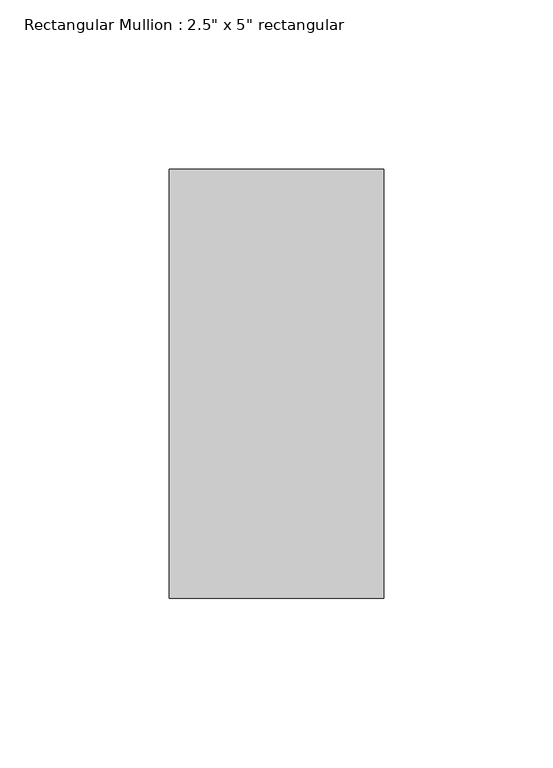
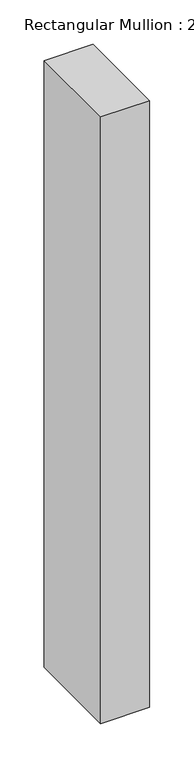
"""IFC4 building model written with IfcOpenShell, lengths in millimetres: member geometry."""

from ifc_helpers import new_model, si_unit, frame, origin, place, context, project, spatial, polyline, outline, extrude, source, transform, mapped, element, save


def member_2ad165f7(model_context):
    return source(origin(), model_context, "Body", "SweptSolid", [
        extrude(outline(polyline([(0.0, 63.5), (0.0, -63.5), (-63.5, -63.5), (-63.5, 63.5), (0.0, 63.5)])), frame((0.0, 0.0, -832.4388769), z_axis=(0.0, 0.0, 1.0), x_axis=(1.0, 0.0, 0.0)), (0.0, 0.0, 1.0), 832.4388769),
    ])


if __name__ == "__main__":
    model = new_model("IFC4")
    model_context = context("Model", 3, world=origin())
    ifc_project = project(units=[si_unit("LENGTHUNIT", "METRE", prefix="MILLI")], contexts=[model_context])
    site = spatial("IfcSite", under=ifc_project)
    building = spatial("IfcBuilding", under=site)
    placement = place(None, origin())
    member_shape = member_2ad165f7(model_context)
    element("IfcMember", 1, ObjectType="Rectangular Mullion : 2.5\" x 5\" rectangular", at=placement, inside=building, context=model_context, shape_type="MappedRepresentation", body=[
        mapped(member_shape, transform((0.0, 0.0, 0.0), x_axis=(1.0, 0.0, 0.0), y_axis=(0.0, 1.0, 0.0), z_axis=(0.0, 0.0, 1.0))),
    ])
    save(model, "model.ifc")

# Revit data of these elements
# Type "Rectangular Mullion : 2.5\" x 5\" rectangular"
#   built-in parameter 1007304 = 0.416667 (stored number, unit not read)
#   built-in parameter 1007301 = 0.104167 (stored number, unit not read)
#   built-in parameter 1007300 = 0.104167 (stored number, unit not read)
# Element 1 (IfcMember, "Rectangular Mullion : 2.5\" x 5\" rectangular")
#   Materials on its faces: "Aluminum"
# Materials
#   "Aluminum": class "Metal", colour RGB 247 247 247, transparency 0, Description = "Aluminum 6061", Cost = 0
